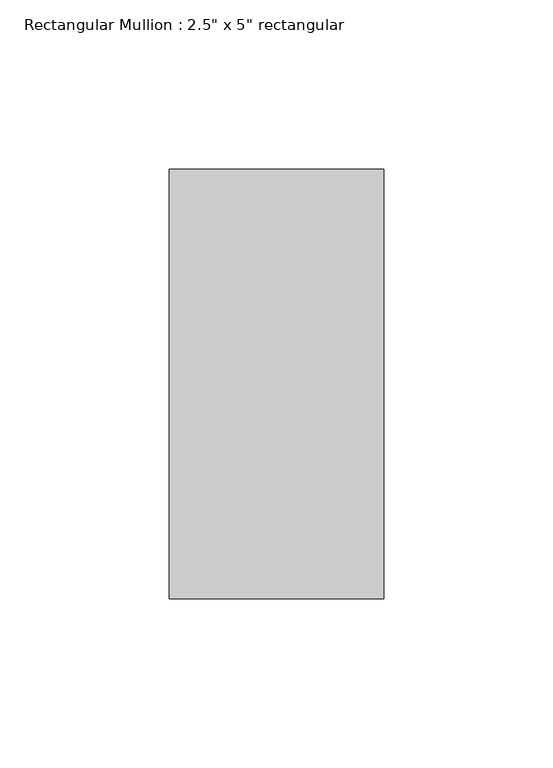
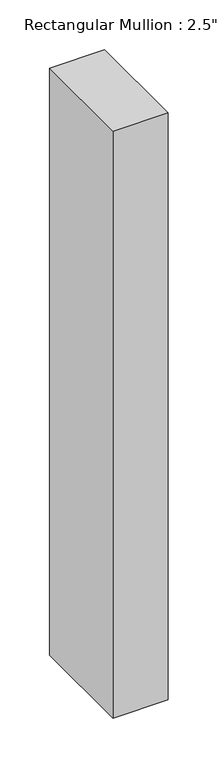
"""IFC4 building model written with IfcOpenShell, lengths in millimetres: member geometry."""

from ifc_helpers import new_model, si_unit, frame, origin, place, context, project, spatial, polyline, outline, extrude, source, transform, mapped, element, save


def member_7007ad49(model_context):
    return source(origin(), model_context, "Body", "SweptSolid", [
        extrude(outline(polyline([(0.0, 63.5), (0.0, -63.5), (-63.5, -63.5), (-63.5, 63.5), (0.0, 63.5)])), frame((0.0, 0.0, -717.55), z_axis=(0.0, 0.0, 1.0), x_axis=(1.0, 0.0, 0.0)), (0.0, 0.0, 1.0), 717.55),
    ])


if __name__ == "__main__":
    model = new_model("IFC4")
    model_context = context("Model", 3, world=origin())
    ifc_project = project(units=[si_unit("LENGTHUNIT", "METRE", prefix="MILLI")], contexts=[model_context])
    site = spatial("IfcSite", under=ifc_project)
    building = spatial("IfcBuilding", under=site)
    placement = place(None, origin())
    member_shape = member_7007ad49(model_context)
    element("IfcMember", 1, ObjectType="Rectangular Mullion : 2.5\" x 5\" rectangular", at=placement, inside=building, context=model_context, shape_type="MappedRepresentation", body=[
        mapped(member_shape, transform((0.0, 0.0, 0.0), x_axis=(1.0, 0.0, 0.0), y_axis=(0.0, 1.0, 0.0), z_axis=(0.0, 0.0, 1.0))),
    ])
    save(model, "model.ifc")

# Revit data of these elements
# Type "Rectangular Mullion : 2.5\" x 5\" rectangular"
#   built-in parameter 1007304 = 0.416667 (stored number, unit not read)
#   built-in parameter 1007301 = 0.104167 (stored number, unit not read)
#   built-in parameter 1007300 = 0.104167 (stored number, unit not read)
# Element 1 (IfcMember, "Rectangular Mullion : 2.5\" x 5\" rectangular")
#   Materials on its faces: "Door - Frame"
# Materials
#   "Door - Frame": colour RGB 118 70 51, transparency 0, Cost = 0
